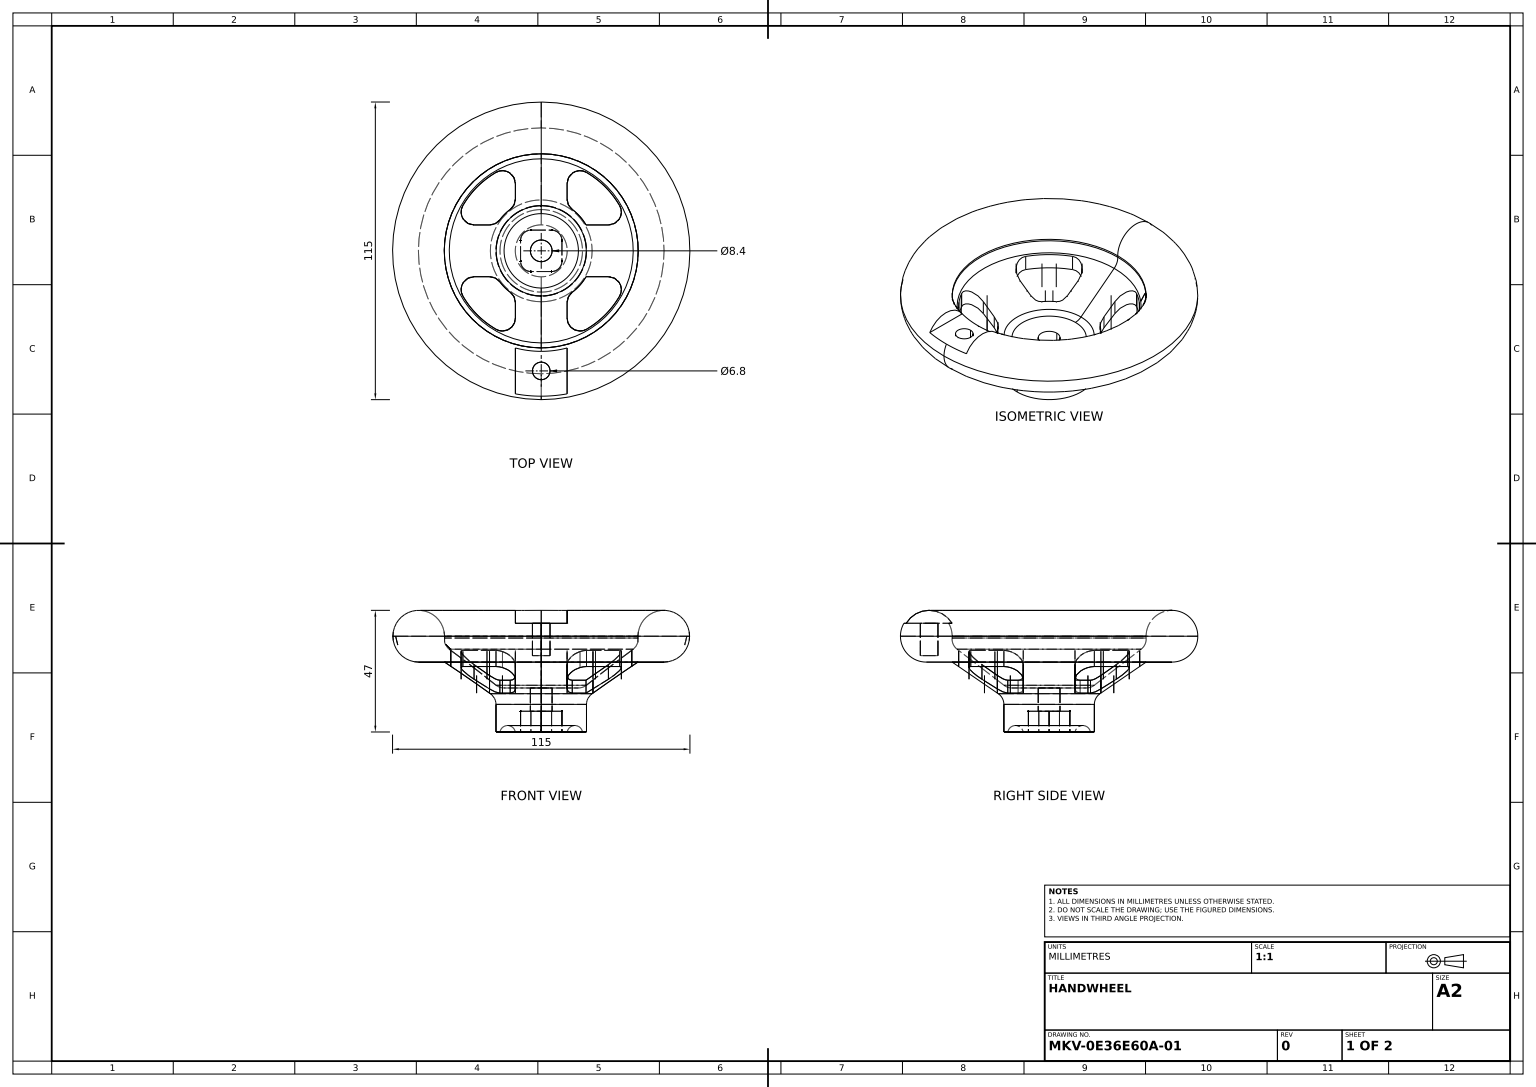
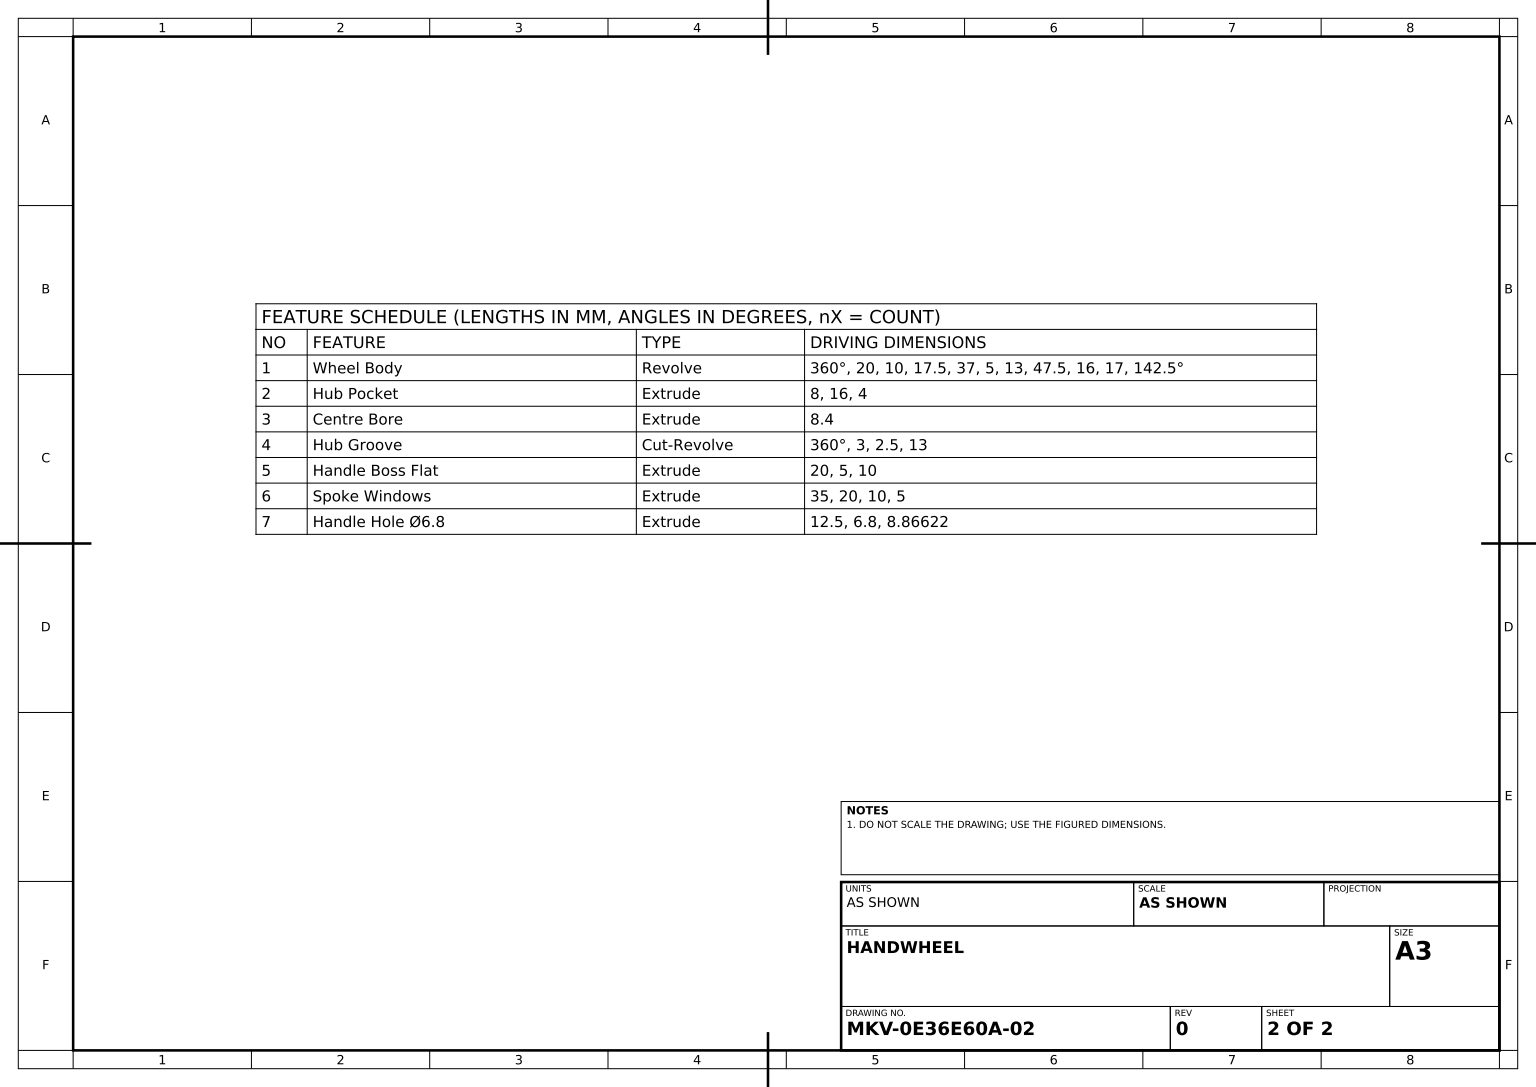
SolidWorks part; units mm, degrees
material "Plain Carbon Steel"
ref_plane "Front Plane" through (0, 0, 0) normal (0, 0, 1) x (1, 0, 0)
ref_plane "Top Plane" through (0, 0, 0) normal (0, 1, 0) x (1, 0, 0)
ref_plane "Right Plane" through (0, 0, 0) normal (1, 0, 0) x (0, 0, -1)
sketch "Wheel Body Profile" plane through (0, 0, 0) normal (0, 0, 1) x (1, 0, 0)
  line L0 (0, -10) -> (10, -10)
  line L1 (11.9163, -5.0212) -> (30.0623, -18.9647)
  line L2 (33.1088, -20) -> (47.5, -20)
  line L3 (47.5, -20) -> (47.5, -37)
  line L6 (47.5, -37) -> (47.5, 33.6587) construction
  line L7 (47.5, -37) -> (30, -37)
  line L8 (30, -37) -> (30, -26.3318)
  line L9 (27.825, -22.2064) -> (10, -10)
  arc A0 (9.9752, -0.7043) -> (0, -10) centre (0, 0) ccw
  arc A2 (30, -26.3318) -> (27.825, -22.2064) centre (25, -26.3318) ccw
  arc A3 (33.1088, -20) -> (30.0623, -18.9647) centre (33.1088, -15) cw
  arc A4 (9.9752, -0.7043) -> (11.9163, -5.0212) centre (14.9627, -1.0565) ccw
  point P8 (0, 10)
  point P9 (31.5, -19.7341)
  point P10 (29.423, -24)
  point P20 (30, -23.6958)
  dimension "D1" = 20
  dimension "D2" = 47.5
  dimension "D7" = 17.5
  dimension "D10" = 5
  dimension "D12" = 5
  dimension "D5" = 16
  dimension "D6" = 13
  dimension "D4" = 5
  dimension "D11" = 142.461
  dimension "D3" = 10
  dimension "D8" = 17
  dimension "D9" = 37
revolve "Wheel Body" add sketch "Wheel Body Profile" angle 360 about L6
sketch "Hub Pocket Sketch" plane through (0, -37, 0) normal (0, -1, 0) x (1, 0, 0)
  line L1 (43.5, -8) -> (51.5, -8)
  line L2 (39.5, -4) -> (39.5, 4)
  line L3 (43.5, 8) -> (51.5, 8)
  line L4 (55.5, -4) -> (55.5, 4)
  line L5 (39.5, -8) -> (55.5, 8) construction
  line L6 (39.5, 8) -> (55.5, -8) construction
  arc A0 (43.5, -8) -> (39.5, -4) centre (43.5, -4) cw
  arc A1 (51.5, -8) -> (55.5, -4) centre (51.5, -4) ccw
  arc A2 (55.5, 4) -> (51.5, 8) centre (51.5, 4) ccw
  arc A3 (39.5, 4) -> (43.5, 8) centre (43.5, 4) cw
  point P0 (47.5, 0)
  dimension "D3" = 4
  dimension "D1" = 16
  dimension "D2" = 16
extrude "Hub Pocket" cut sketch "Hub Pocket Sketch" against normal blind 8
sketch "Centre Bore Sketch" plane through (0, -37, 0) normal (0, -1, 0) x (1, 0, 0)
  circle A0 centre (47.5, 0) radius 4.2
  dimension "D1" = 8.4
extrude "Centre Bore" cut sketch "Centre Bore Sketch" against normal through all
sketch "Hub Groove Profile" plane through (0, 0, 0) normal (0, 0, 1) x (1, 0, 0)
  line L0 (30, -37) -> (65, -37) construction
  line L2 (47.5, -24.2541) -> (47.5, -61.7738) construction
  line L3 (31.542, -37) -> (37.458, -37)
  arc A0 (37.458, -37) -> (31.542, -37) centre (34.5, -37.5) ccw
  point P4 (47.5, -37)
  point P8 (34.5, -34.5)
  dimension "D1" = 3
  dimension "D2" = 2.5
  dimension "D3" = 13
revolve "Hub Groove" cut sketch "Hub Groove Profile" angle 360 about L2
sketch "Handle Boss Flat Sketch" plane through (0, 0, 0) normal (0, 0, 1) x (1, 0, 0)
  line L0 (47.5, -37) -> (47.5, 25.6926) construction
  line L1 (30, -37) -> (65, -37) construction
  line L2 (37.5, 10) -> (37.5, 5)
  line L3 (95, 10) -> (0, 10) construction
  line L4 (37.5, 10) -> (57.5, 10)
  line L5 (37.5, 5) -> (57.5, 5)
  line L6 (57.5, 5) -> (57.5, 10)
  dimension "D1" = 20
  dimension "D2" = 5
  dimension "D3" = 10
extrude "Handle Boss Flat" cut sketch "Handle Boss Flat Sketch" along normal through all
sketch "Spoke Windows Sketch" plane through (0, 0, 0) normal (0, 1, 0) x (1, 0, 0)
  line L0 (47.5, 85.2293) -> (47.5, -90.2202) construction
  line L1 (-24.4259, 0) -> (127.7338, 0) construction
  line L2 (21.5192, 10) -> (27.5, 10)
  line L3 (64.8205, 10) -> (73.4808, 10)
  line L4 (37.5, 20) -> (37.5, 25.9808)
  line L5 (57.5, 20) -> (57.5, 25.9808)
  line L6 (64.8205, -10) -> (73.4808, -10)
  line L7 (57.5, -20) -> (57.5, -25.9808)
  line L8 (21.5192, -10) -> (27.5, -10)
  line L9 (37.5, -20) -> (37.5, -25.9808)
  arc A1 (17.1891, -17.5) -> (30, -30.3109) centre (47.5, 0) ccw
  arc A2 (35.5, 16) -> (31.5, 12) centre (47.5, 0) ccw
  arc A3 (30, 30.3109) -> (17.1891, 17.5) centre (47.5, 0) ccw
  arc A4 (31.5, -12) -> (67.5, 0) centre (47.5, 0) ccw
  arc A5 (37.5, 25.9808) -> (30, 30.3109) centre (32.5, 25.9808) ccw
  arc A6 (35.5, 16) -> (37.5, 20) centre (32.5, 20) ccw
  arc A7 (27.5, 10) -> (31.5, 12) centre (27.5, 15) ccw
  arc A8 (21.5192, 10) -> (17.1891, 17.5) centre (21.5192, 15) cw
  arc A9 (64.8205, 10) -> (59.5, 16) centre (47.5, 0) ccw
  arc A10 (77.8109, 17.5) -> (65, 30.3109) centre (47.5, 0) ccw
  arc A11 (77.8109, 17.5) -> (73.4808, 10) centre (73.4808, 15) cw
  arc A12 (57.5, 25.9808) -> (65, 30.3109) centre (62.5, 25.9808) cw
  arc A13 (59.5, 16) -> (57.5, 20) centre (62.5, 20) cw
  arc A14 (64.8205, -10) -> (59.5, -16) centre (47.5, 0) cw
  arc A15 (77.8109, -17.5) -> (73.4808, -10) centre (73.4808, -15) ccw
  arc A16 (77.8109, -17.5) -> (65, -30.3109) centre (47.5, 0) cw
  arc A17 (57.5, -25.9808) -> (65, -30.3109) centre (62.5, -25.9808) ccw
  arc A18 (59.5, -16) -> (57.5, -20) centre (62.5, -20) ccw
  arc A19 (35.5, -16) -> (31.5, -12) centre (47.5, 0) cw
  arc A20 (27.5, -10) -> (31.5, -12) centre (27.5, -15) cw
  arc A21 (21.5192, -10) -> (17.1891, -17.5) centre (21.5192, -15) ccw
  arc A22 (30, -30.3109) -> (17.1891, -17.5) centre (47.5, 0) cw
  arc A23 (37.5, -25.9808) -> (30, -30.3109) centre (32.5, -25.9808) cw
  arc A24 (35.5, -16) -> (37.5, -20) centre (32.5, -20) cw
  arc A25 (65, -30.3109) -> (82.5, 0) centre (47.5, 0) ccw
  point P19 (37.5, 33.541)
  point P30 (81.041, 10)
  dimension "D1" = 35
  dimension "D2" = 20
  dimension "D4" = 5
  dimension "D6" = 5
  dimension "D3" = 10
  dimension "D5" = 10
  dimension "D7" = 10
  dimension "D8" = 10
extrude "Spoke Windows" cut sketch "Spoke Windows Sketch" against normal through all contours A24 A4 A20 L8 A21 A1 A23 L9 | A8 L2 A7 A2 A6 L4 A5 A3 | A13 A9 L3 A11 A10 A12 L5 | A4 A18 L7 A17 A16 A15 L6
sketch "Handle Hole Sketch" plane through (0, 5, 0) normal (0, 1, 0) x (1, 0, 0)
  line L0 (47.5, 0) -> (47.5, -72.1459) construction
  circle A0 centre (47.5, -46.3966) radius 3.4
  dimension "D1" = 6.8
  dimension "D2" = 8.8662
extrude "Handle Hole Ø6.8" cut sketch "Handle Hole Sketch" against normal blind 12.5
